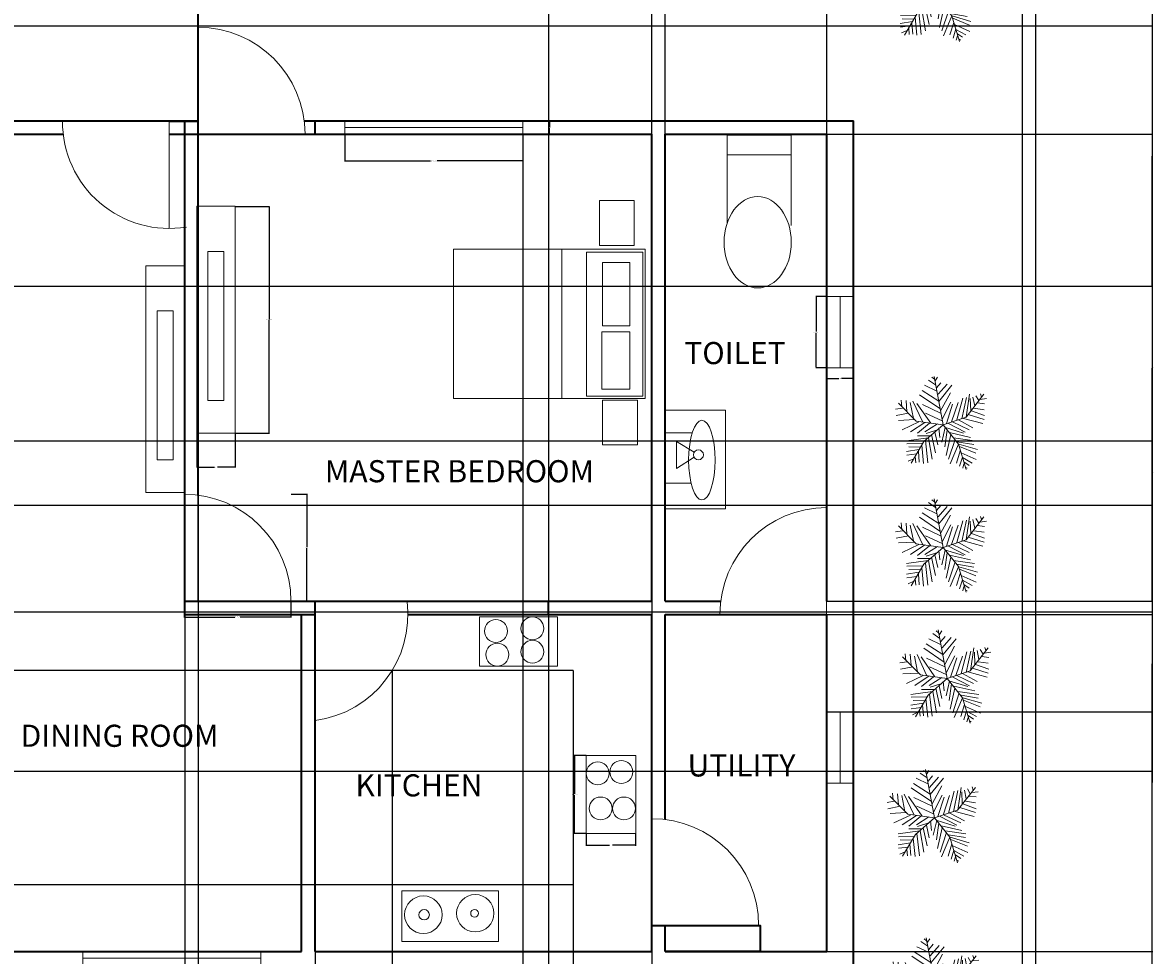
# Model space of a CAD drawing. Units: inches. Extents: x -86 to 773, y -188 to 560.
# Tile 5 of 6: x 392 to 773, y 85 to 400. Entities that reach past the tile are written whole.
import ezdxf

# ---------------------------------------------------------------- set-up
doc = ezdxf.new("R2010")
doc.units = ezdxf.units.IN
doc.header["$MEASUREMENT"] = 0
for name, color, linetype, lineweight in [('A-ANNO-DIMS', 2, 'Continuous', 18), ('A-AREA-IDEN', 7, 'Continuous', 25), ('A-DOOR', 7, 'Continuous', 18), ('A-EQPM', 8, 'Continuous', 18), ('A-FLOR-CASE', 8, 'Continuous', 18), ('A-FLOR-FIXT', 8, 'Continuous', 18), ('A-FURN', 8, 'Continuous', 18), ('A-GLAZ', 7, 'Continuous', 18), ('A-WALL', 7, 'Continuous', 35), ('C-PROP', 7, 'Continuous', 25), ('L-HRDS', 7, 'Continuous', 18), ('L-PLNT-TREE', 8, 'Continuous', 9)]:
    doc.layers.add(name, color=color, linetype=linetype, lineweight=lineweight)
doc.styles.get("Standard").update_dxf_attribs({"font": 'arial.ttf'})
doc.dimstyles.get("Standard").update_dxf_attribs({"dimtxt": 0.18, "dimasz": 0.18, "dimexe": 0.18, "dimexo": 0.0625, "dimgap": 0.09, "dimtad": 0, "dimtih": 1, "dimtoh": 1, "dimdec": 4, "dimzin": 0, "dimdsep": 46, "dimtxsty": 'Standard', "dimcen": 0.09, "dimadec": 0, "dimazin": 0, "dimtfac": 1, "dimtdec": 4, "dimtofl": 0, "dimtmove": 0, "dimatfit": 3, "dimfxl": 1, "dimtolj": 1, "dimtzin": 0, "dimarcsym": 0})

# ---------------------------------------------------------------- blocks, each defined once
blk = doc.blocks.new('Trees - Metric')
for p, q in [((-258.7244, 1362.456), (-332.3336, 1421.4348)), ((0, 0), (-266.7, 1447.8)), ((-231.1146, 1315.2628), (-166.7002, 1421.4348)), ((-129.8956, 713.6638), (-626.7704, 1032.1544)), ((-185.1152, 1008.5578), (-553.1612, 1185.4942)), ((-221.9198, 1197.3052), (-433.5526, 1338.8594)), ((-194.31, 1102.9442), (-65.4812, 1256.284)), ((-148.3106, 914.1968), (118.5418, 1220.9018)), ((-129.8956, 701.8528), (265.7602, 1185.4942)), ((-1234.059, 536.7274), (-1252.4486, 737.2604)), ((-1105.2302, 725.4494), (-1077.6458, 395.1732)), ((-902.8176, 713.6638), (-617.5756, 100.2538)), ((-93.091, 489.5342), (-700.3796, 902.3858)), ((-74.7014, 418.7444), (219.7608, 961.39)), ((-28.6766, 171.0436), (228.9556, 678.2816)), ((412.9786, 147.447), (587.8068, 796.2392)), ((560.197, 182.8292), (698.2206, 819.8358)), ((685.8, 228.6), (1219.2, 914.4)), ((689.0258, 230.0224), (790.2448, 914.1968)), ((808.6344, 784.4282), (827.0494, 418.7444)), ((891.4384, 831.6214), (946.658, 572.1096)), ((983.4626, 867.0036), (1066.2666, 725.4494)), ((1112.2914, 760.8316), (1296.3144, 784.4282)), ((1121.4862, 925.9824), (1149.0706, 831.6214)), ((-1206.4492, 501.3198), (-1418.082, 465.9376)), ((-1031.621, 347.98), (-1399.667, 277.1902)), ((-800.1, 114.3), (-1333.5, 647.7)), ((-976.4268, 666.4706), (-884.4026, 194.6402)), ((-369.1382, 53.086), (-783.1836, 642.874)), ((-617.5756, 607.4918), (-74.7014, 347.98)), ((-525.5514, 347.98), (-28.6766, 123.8504)), ((100.1268, 41.275), (284.1498, 619.2774)), ((256.5654, 88.4682), (449.7832, 666.4706)), ((845.439, 418.7444), (1241.0948, 277.1902)), ((919.0482, 501.3198), (1222.6798, 454.152)), ((1029.462, 654.685), (1241.0948, 631.0884)), ((-847.598, 159.2326), (-1326.0578, 135.636)), ((-718.7946, 88.4682), (-1215.644, -147.447)), ((-543.9664, 76.6572), (-967.2066, -206.4512)), ((0, 0), (-800.1, 114.3)), ((-405.9428, 53.086), (-764.794, -241.8334)), ((0, 0), (-571.5, -495.3)), ((-166.7002, 29.4894), (-543.9664, -206.4512)), ((0, 0), (685.8, 228.6)), ((0, 0), (457.2, -571.5)), ((164.5412, 41.275), (661.416, -218.2368)), ((284.1498, 88.4682), (781.0246, -147.447)), ((458.978, 147.447), (891.4384, -88.4682)), ((615.4166, 194.6402), (1185.8752, 41.275)), ((753.4148, 312.5978), (1222.6798, 159.2326)), ((-387.5278, -324.4088), (-764.794, -324.4088)), ((-166.7002, -147.447), (-507.1618, -253.619)), ((-341.5284, -289.0012), (-221.9198, -831.6214)), ((-240.3094, -218.2368), (-157.5054, -595.7062)), ((-120.7008, -88.4682), (-93.091, -371.5766)), ((63.3222, -76.6826), (-37.8714, -513.1308)), ((44.9326, -64.897), (615.4166, -241.8334)), ((127.7366, -159.258), (54.1274, -654.685)), ((228.9556, -289.0012), (90.932, -914.1968)), ((192.151, -230.0224), (817.8292, -371.5766)), ((-442.7474, -383.3876), (-1086.8406, -477.7486)), ((-617.5756, -548.5384), (-1077.6458, -560.324)), ((-681.9646, -666.496), (-1022.4262, -654.685)), ((-571.5, -495.3), (-952.5, -1143)), ((-635.9652, -607.5172), (-580.771, -1150.1374)), ((-525.5514, -465.963), (-451.9422, -1126.5408)), ((-433.5526, -383.3876), (-323.1134, -1020.3688)), ((357.759, -430.5554), (164.5412, -1020.3688)), ((458.978, -572.1096), (210.5406, -1161.923)), ((311.7596, -383.3876), (937.4378, -477.7486)), ((412.9786, -501.3452), (919.0482, -583.9206)), ((457.2, -571.5), (685.8, -1333.5)), ((468.1982, -572.1096), (1029.462, -737.2604)), ((486.5878, -642.8994), (983.4626, -843.4324)), ((-718.7946, -737.2604), (-1086.8406, -796.2392)), ((-783.1836, -867.029), (-1077.6458, -902.4112)), ((-875.2078, -1008.5832), (-1040.8412, -1079.3476)), ((-829.2084, -937.7934), (-810.7934, -1126.5408)), ((-737.1842, -784.4536), (-709.5744, -1114.7298)), ((514.1976, -772.6426), (403.7838, -1138.3264)), ((578.612, -961.39), (495.7826, -1232.7128)), ((541.8074, -831.6214), (992.6574, -1032.1544)), ((578.612, -973.1756), (873.0488, -1138.3264)), ((624.6114, -1161.923), (587.8068, -1291.6916)), ((624.6114, -1102.9442), (781.0246, -1209.1162)), ((679.8056, -1268.095), (716.6102, -1291.6916))]:
    blk.add_line(p, q)
blk = doc.blocks.new('BED-DOUBLE-NIGHTSTANDS')
blk.add_line((16.69, 36.48), (66.76, 36.48))
for points in [[(16.43, 64.62), (66.76, 64.62), (66.76, 0), (16.43, 0)], [(17.47, 63.83), (65.98, 63.83), (65.98, 44.81), (17.47, 44.81)], [(82.41, 62.01), (67.29, 62.01), (67.29, 50.29), (82.41, 50.29)], [(15.13, 60.97), (0, 60.97), (0, 49.24), (15.13, 49.24)], [(20.86, 59.41), (42.25, 59.41), (42.25, 50.29), (20.86, 50.29)], [(44.34, 59.41), (63.63, 59.41), (63.63, 50.03), (44.34, 50.03)]]:
    blk.add_lwpolyline(points, close=True)
blk = doc.blocks.new('DOOR-SWING-36')
for p, q in [((0, 0), (0, 36)), ((36, 0), (0, 0))]:
    blk.add_line(p, q)
blk.add_arc((0, 0), 36, 0, 90)
blk = doc.blocks.new('DOOR-LEAF-36')
blk.add_line((0, 0), (36, 0))
blk.add_arc((36, 0), 36, 90, 180)
blk = doc.blocks.new('WIN-24-W9')
for p, q in [((0, 9), (0, 0)), ((24, 9), (24, 0)), ((24, 4.5), (0, 4.5))]:
    blk.add_line(p, q)
blk = doc.blocks.new('WIN-60-W4_5')
for p, q in [((0, 4.5), (0, 0)), ((60, 4.5), (60, 0)), ((60, 2.25), (0, 2.25))]:
    blk.add_line(p, q)
blk = doc.blocks.new('COOKTOP-4-BURNER')
blk.add_lwpolyline([(0, 16.64), (26.31, 16.64), (26.31, 0), (0, 0)], close=True)
for centre in [(5.55, 11.81), (17.86, 12.69), (6.03, 3.86), (17.86, 4.82)]:
    blk.add_circle(centre, 3.86)
blk = doc.blocks.new('MEDIA-CONSOLE')
for points in [[(0, 76.46), (12.95, 76.46), (12.95, 0), (0, 0)], [(3.81, 61.24), (9.14, 61.24), (9.14, 11.03), (3.81, 11.03)]]:
    blk.add_lwpolyline(points, close=True)
blk = doc.blocks.new('BASIN-TAP')
blk.add_lwpolyline([(3.11, 5.27), (9.09, 9.11), (9.09, 0), (3.06, 3.55)])
blk.add_circle((1.66, 4.45), 1.66)
blk = doc.blocks.new('*D25')
at = {"layer": 'A-ANNO-DIMS', "color": 0, "lineweight": -2, "transparency": 16777216}
for p, q in [((446.27, 204.59), (446.27, 199.07)), ((482.27, 204.59), (482.27, 199.07)), ((446.45, 199.25), (463.34, 199.25)), ((482.09, 199.25), (465.21, 199.25))]:
    blk.add_line(p, q, dxfattribs=at)
at = {"layer": 'A-ANNO-DIMS', "color": 0, "transparency": 16777216}
for points in [[(446.45, 199.28), (446.45, 199.22), (446.27, 199.25)], [(482.09, 199.28), (482.09, 199.22), (482.27, 199.25)]]:
    blk.add_solid(points, dxfattribs=at)
at = {"layer": 'Defpoints', "color": 0, "transparency": 16777216}
for p in [(446.27, 204.65), (482.27, 204.65), (482.27, 199.25)]:
    blk.add_point(p, dxfattribs=at)
at = {"layer": 'A-ANNO-DIMS', "color": 0, "transparency": 16777216, "insert": (464.27, 199.25), "char_height": 0.18, "attachment_point": 5}
blk.add_mtext('\\A1;DOOR 36 TYP.', dxfattribs=at)
blk = doc.blocks.new('*D26')
at = {"layer": 'A-ANNO-DIMS', "color": 0, "lineweight": -2, "transparency": 16777216}
for p, q in [((482.34, 240.65), (487.85, 240.65)), ((487.67, 240.47), (487.67, 222.83)), ((487.67, 204.83), (487.67, 222.47)), ((482.34, 204.65), (487.85, 204.65))]:
    blk.add_line(p, q, dxfattribs=at)
at = {"layer": 'A-ANNO-DIMS', "color": 0, "transparency": 16777216}
for points in [[(487.64, 240.47), (487.7, 240.47), (487.67, 240.65)], [(487.64, 204.83), (487.7, 204.83), (487.67, 204.65)]]:
    blk.add_solid(points, dxfattribs=at)
at = {"layer": 'Defpoints', "color": 0, "transparency": 16777216}
for p in [(482.27, 240.65), (487.67, 240.65), (482.27, 204.65)]:
    blk.add_point(p, dxfattribs=at)
at = {"layer": 'A-ANNO-DIMS', "color": 0, "transparency": 16777216, "insert": (487.67, 222.65), "char_height": 0.18, "attachment_point": 5}
blk.add_mtext('\\A1;36 TYP.', dxfattribs=at)
blk = doc.blocks.new('*D27')
at = {"layer": 'A-ANNO-DIMS', "color": 0, "lineweight": -2, "transparency": 16777216}
for p, q in [((662.95, 307.3), (659.23, 307.3)), ((659.41, 307.12), (659.41, 295.48)), ((659.41, 283.48), (659.41, 295.11)), ((662.95, 283.3), (659.23, 283.3))]:
    blk.add_line(p, q, dxfattribs=at)
at = {"layer": 'A-ANNO-DIMS', "color": 0, "transparency": 16777216}
for points in [[(659.38, 307.12), (659.44, 307.12), (659.41, 307.3)], [(659.38, 283.48), (659.44, 283.48), (659.41, 283.3)]]:
    blk.add_solid(points, dxfattribs=at)
at = {"layer": 'Defpoints', "color": 0, "transparency": 16777216}
for p in [(659.41, 307.3), (663.01, 307.3), (663.01, 283.3)]:
    blk.add_point(p, dxfattribs=at)
at = {"layer": 'A-ANNO-DIMS', "color": 0, "transparency": 16777216, "insert": (659.41, 295.3), "char_height": 0.18, "attachment_point": 5}
blk.add_mtext('\\A1;WINDOW 24 TYP.', dxfattribs=at)
blk = doc.blocks.new('*D28')
at = {"layer": 'A-ANNO-DIMS', "color": 0, "lineweight": -2, "transparency": 16777216}
for p, q in [((663.01, 283.23), (663.01, 279.52)), ((672.01, 283.23), (672.01, 279.52)), ((663.19, 279.7), (667.05, 279.7)), ((671.83, 279.7), (667.97, 279.7))]:
    blk.add_line(p, q, dxfattribs=at)
at = {"layer": 'A-ANNO-DIMS', "color": 0, "transparency": 16777216}
for points in [[(663.19, 279.73), (663.19, 279.67), (663.01, 279.7)], [(671.83, 279.73), (671.83, 279.67), (672.01, 279.7)]]:
    blk.add_solid(points, dxfattribs=at)
at = {"layer": 'Defpoints', "color": 0, "transparency": 16777216}
for p in [(663.01, 283.3), (672.01, 283.3), (663.01, 279.7)]:
    blk.add_point(p, dxfattribs=at)
at = {"layer": 'A-ANNO-DIMS', "color": 0, "transparency": 16777216, "insert": (667.51, 279.7), "char_height": 0.18, "attachment_point": 5}
blk.add_mtext('\\A1;9 TYP.', dxfattribs=at)
blk = doc.blocks.new('*D29')
at = {"layer": 'A-ANNO-DIMS', "color": 0, "lineweight": -2, "transparency": 16777216}
for p, q in [((500.48, 361.95), (500.48, 352.83)), ((560.48, 361.95), (560.48, 352.83)), ((500.66, 353.01), (529.36, 353.01)), ((560.3, 353.01), (531.59, 353.01))]:
    blk.add_line(p, q, dxfattribs=at)
at = {"layer": 'A-ANNO-DIMS', "color": 0, "transparency": 16777216}
for points in [[(500.66, 353.04), (500.66, 352.98), (500.48, 353.01)], [(560.3, 353.04), (560.3, 352.98), (560.48, 353.01)]]:
    blk.add_solid(points, dxfattribs=at)
at = {"layer": 'Defpoints', "color": 0, "transparency": 16777216}
for p in [(500.48, 362.01), (560.48, 362.01), (560.48, 353.01)]:
    blk.add_point(p, dxfattribs=at)
at = {"layer": 'A-ANNO-DIMS', "color": 0, "transparency": 16777216, "insert": (530.48, 353.01), "char_height": 0.18, "attachment_point": 5}
blk.add_mtext('\\A1;WINDOW 60 TYP.', dxfattribs=at)
blk = doc.blocks.new('*D30')
at = {"layer": 'A-ANNO-DIMS', "color": 0, "lineweight": -2, "transparency": 16777216}
for p, q in [((560.54, 366.51), (569.66, 366.51)), ((569.48, 366.33), (569.48, 364.44)), ((569.48, 362.19), (569.48, 364.08)), ((560.54, 362.01), (569.66, 362.01))]:
    blk.add_line(p, q, dxfattribs=at)
at = {"layer": 'A-ANNO-DIMS', "color": 0, "transparency": 16777216}
for points in [[(569.45, 366.33), (569.51, 366.33), (569.48, 366.51)], [(569.45, 362.19), (569.51, 362.19), (569.48, 362.01)]]:
    blk.add_solid(points, dxfattribs=at)
at = {"layer": 'Defpoints', "color": 0, "transparency": 16777216}
for p in [(560.48, 366.51), (569.48, 366.51), (560.48, 362.01)]:
    blk.add_point(p, dxfattribs=at)
at = {"layer": 'A-ANNO-DIMS', "color": 0, "transparency": 16777216, "insert": (569.48, 364.26), "char_height": 0.18, "attachment_point": 5}
blk.add_mtext('\\A1;5 TYP.', dxfattribs=at)
blk = doc.blocks.new('*D39')
at = {"layer": 'A-ANNO-DIMS', "color": 0, "lineweight": -2, "transparency": 16777216}
for p, q in [((581.81, 152.57), (577.75, 152.57)), ((577.93, 152.39), (577.93, 139.6)), ((577.93, 126.45), (577.93, 139.24)), ((581.81, 126.27), (577.75, 126.27))]:
    blk.add_line(p, q, dxfattribs=at)
at = {"layer": 'A-ANNO-DIMS', "color": 0, "transparency": 16777216}
for points in [[(577.9, 152.39), (577.96, 152.39), (577.93, 152.57)], [(577.9, 126.45), (577.96, 126.45), (577.93, 126.27)]]:
    blk.add_solid(points, dxfattribs=at)
at = {"layer": 'Defpoints', "color": 0, "transparency": 16777216}
for p in [(581.87, 152.57), (577.93, 126.27), (581.87, 126.27)]:
    blk.add_point(p, dxfattribs=at)
at = {"layer": 'A-ANNO-DIMS', "color": 0, "transparency": 16777216, "insert": (577.93, 139.42), "char_height": 0.18, "attachment_point": 5}
blk.add_mtext('\\A1;COOKTOP 26 TYP.', dxfattribs=at)
blk = doc.blocks.new('*D40')
at = {"layer": 'A-ANNO-DIMS', "color": 0, "lineweight": -2, "transparency": 16777216}
for p, q in [((581.87, 126.21), (581.87, 122.14)), ((598.51, 126.21), (598.51, 122.14)), ((582.05, 122.32), (589.67, 122.32)), ((598.33, 122.32), (590.71, 122.32))]:
    blk.add_line(p, q, dxfattribs=at)
at = {"layer": 'A-ANNO-DIMS', "color": 0, "transparency": 16777216}
for points in [[(582.05, 122.35), (582.05, 122.29), (581.87, 122.32)], [(598.33, 122.35), (598.33, 122.29), (598.51, 122.32)]]:
    blk.add_solid(points, dxfattribs=at)
at = {"layer": 'Defpoints', "color": 0, "transparency": 16777216}
for p in [(581.87, 126.27), (598.51, 126.27), (598.51, 122.32)]:
    blk.add_point(p, dxfattribs=at)
at = {"layer": 'A-ANNO-DIMS', "color": 0, "transparency": 16777216, "insert": (590.19, 122.32), "char_height": 0.18, "attachment_point": 5}
blk.add_mtext('\\A1;17 TYP.', dxfattribs=at)
blk = doc.blocks.new('*D41')
at = {"layer": 'A-ANNO-DIMS', "color": 0, "lineweight": -2, "transparency": 16777216}
for p, q in [((463.51, 337.71), (475.09, 337.71)), ((474.91, 337.53), (474.91, 299.67)), ((474.91, 261.44), (474.91, 299.3)), ((463.51, 261.26), (475.09, 261.26))]:
    blk.add_line(p, q, dxfattribs=at)
at = {"layer": 'A-ANNO-DIMS', "color": 0, "transparency": 16777216}
for points in [[(474.88, 337.53), (474.94, 337.53), (474.91, 337.71)], [(474.88, 261.44), (474.94, 261.44), (474.91, 261.26)]]:
    blk.add_solid(points, dxfattribs=at)
at = {"layer": 'Defpoints', "color": 0, "transparency": 16777216}
for p in [(463.44, 337.71), (474.91, 337.71), (463.44, 261.26)]:
    blk.add_point(p, dxfattribs=at)
at = {"layer": 'A-ANNO-DIMS', "color": 0, "transparency": 16777216, "insert": (474.91, 299.48), "char_height": 0.18, "attachment_point": 5}
blk.add_mtext('\\A1;CONSOLE 76 TYP.', dxfattribs=at)
blk = doc.blocks.new('*D42')
at = {"layer": 'A-ANNO-DIMS', "color": 0, "lineweight": -2, "transparency": 16777216}
for p, q in [((450.5, 261.19), (450.5, 249.61)), ((463.44, 261.19), (463.44, 249.61)), ((450.68, 249.79), (456.45, 249.79)), ((463.26, 249.79), (457.49, 249.79))]:
    blk.add_line(p, q, dxfattribs=at)
at = {"layer": 'A-ANNO-DIMS', "color": 0, "transparency": 16777216}
for points in [[(450.68, 249.82), (450.68, 249.76), (450.5, 249.79)], [(463.26, 249.82), (463.26, 249.76), (463.44, 249.79)]]:
    blk.add_solid(points, dxfattribs=at)
at = {"layer": 'Defpoints', "color": 0, "transparency": 16777216}
for p in [(450.5, 261.26), (463.44, 261.26), (463.44, 249.79)]:
    blk.add_point(p, dxfattribs=at)
at = {"layer": 'A-ANNO-DIMS', "color": 0, "transparency": 16777216, "insert": (456.97, 249.79), "char_height": 0.18, "attachment_point": 5}
blk.add_mtext('\\A1;13 TYP.', dxfattribs=at)
blk = doc.blocks.new('*D46')
at = {"layer": 'A-ANNO-DIMS', "color": 0, "lineweight": -2, "transparency": 16777216}
for p, q in [((733.51, 486.66), (772.88, 486.66)), ((772.7, 486.48), (772.7, 169.55)), ((772.7, -147.74), (772.7, 169.19)), ((733.51, -147.92), (772.88, -147.92))]:
    blk.add_line(p, q, dxfattribs=at)
at = {"layer": 'A-ANNO-DIMS', "color": 0, "transparency": 16777216}
for points in [[(772.67, 486.48), (772.73, 486.48), (772.7, 486.66)], [(772.67, -147.74), (772.73, -147.74), (772.7, -147.92)]]:
    blk.add_solid(points, dxfattribs=at)
at = {"layer": 'Defpoints', "color": 0, "transparency": 16777216}
for p in [(733.45, 486.66), (772.7, 486.66), (733.45, -147.92)]:
    blk.add_point(p, dxfattribs=at)
at = {"layer": 'A-ANNO-DIMS', "color": 0, "transparency": 16777216, "insert": (772.7, 169.37), "char_height": 0.18, "attachment_point": 5}
blk.add_mtext('\\A1;634.6', dxfattribs=at)
blk = doc.blocks.new('*D54')
at = {"layer": 'A-ANNO-DIMS', "color": 0, "lineweight": -2, "transparency": 16777216}
for p, q in [((451.03, 440.67), (451.03, -187.76)), ((569.11, 440.67), (569.11, -187.76)), ((451.21, -187.58), (509.62, -187.58)), ((568.93, -187.58), (510.53, -187.58))]:
    blk.add_line(p, q, dxfattribs=at)
at = {"layer": 'A-ANNO-DIMS', "color": 0, "transparency": 16777216}
for points in [[(451.21, -187.55), (451.21, -187.61), (451.03, -187.58)], [(568.93, -187.55), (568.93, -187.61), (569.11, -187.58)]]:
    blk.add_solid(points, dxfattribs=at)
at = {"layer": 'Defpoints', "color": 0, "transparency": 16777216}
for p in [(451.03, 440.74), (569.11, 440.74), (569.11, -187.58)]:
    blk.add_point(p, dxfattribs=at)
at = {"layer": 'A-ANNO-DIMS', "color": 0, "transparency": 16777216, "insert": (510.07, -187.58), "char_height": 0.18, "attachment_point": 5}
blk.add_mtext('\\A1;118.08', dxfattribs=at)
blk = doc.blocks.new('*D55')
at = {"layer": 'A-ANNO-DIMS', "color": 0, "lineweight": -2, "transparency": 16777216}
for p, q in [((450.97, 440.74), (-85.98, 440.74)), ((-85.8, 440.56), (-85.8, 403.81)), ((-85.8, 366.7), (-85.8, 403.45)), ((450.97, 366.52), (-85.98, 366.52))]:
    blk.add_line(p, q, dxfattribs=at)
at = {"layer": 'A-ANNO-DIMS', "color": 0, "transparency": 16777216}
for points in [[(-85.83, 440.56), (-85.77, 440.56), (-85.8, 440.74)], [(-85.83, 366.7), (-85.77, 366.7), (-85.8, 366.52)]]:
    blk.add_solid(points, dxfattribs=at)
at = {"layer": 'Defpoints', "color": 0, "transparency": 16777216}
for p in [(451.03, 440.74), (-85.8, 366.52), (451.03, 366.52)]:
    blk.add_point(p, dxfattribs=at)
at = {"layer": 'A-ANNO-DIMS', "color": 0, "transparency": 16777216, "insert": (-85.8, 403.63), "char_height": 0.18, "attachment_point": 5}
blk.add_mtext('\\A1;74.22', dxfattribs=at)
blk = doc.blocks.new('*D61')
at = {"layer": 'A-ANNO-DIMS', "color": 0, "lineweight": -2, "transparency": 16777216}
for p, q in [((210.31, 398.62), (772.88, 398.62)), ((772.7, 398.44), (772.7, 354.88)), ((772.7, 310.95), (772.7, 354.52)), ((210.31, 310.77), (772.88, 310.77))]:
    blk.add_line(p, q, dxfattribs=at)
at = {"layer": 'A-ANNO-DIMS', "color": 0, "transparency": 16777216}
for points in [[(772.67, 398.44), (772.73, 398.44), (772.7, 398.62)], [(772.67, 310.95), (772.73, 310.95), (772.7, 310.77)]]:
    blk.add_solid(points, dxfattribs=at)
at = {"layer": 'Defpoints', "color": 0, "transparency": 16777216}
for p in [(210.25, 398.62), (210.25, 310.77), (772.7, 310.77)]:
    blk.add_point(p, dxfattribs=at)
at = {"layer": 'A-ANNO-DIMS', "color": 0, "transparency": 16777216, "insert": (772.7, 354.7), "char_height": 0.18, "attachment_point": 5}
blk.add_mtext('\\A1;87.85', dxfattribs=at)
blk = doc.blocks.new('*D62')
at = {"layer": 'A-ANNO-DIMS', "color": 0, "lineweight": -2, "transparency": 16777216}
for p, q in [((210.33, 201.01), (772.88, 201.01)), ((772.7, 200.83), (772.7, 174.33)), ((772.7, 147.46), (772.7, 173.96)), ((210.31, 147.28), (772.88, 147.28))]:
    blk.add_line(p, q, dxfattribs=at)
at = {"layer": 'A-ANNO-DIMS', "color": 0, "transparency": 16777216}
for points in [[(772.67, 200.83), (772.73, 200.83), (772.7, 201.01)], [(772.67, 147.46), (772.73, 147.46), (772.7, 147.28)]]:
    blk.add_solid(points, dxfattribs=at)
at = {"layer": 'Defpoints', "color": 0, "transparency": 16777216}
for p in [(210.26, 201.01), (210.25, 147.28), (772.7, 147.28)]:
    blk.add_point(p, dxfattribs=at)
at = {"layer": 'A-ANNO-DIMS', "color": 0, "transparency": 16777216, "insert": (772.7, 174.14), "char_height": 0.18, "attachment_point": 5}
blk.add_mtext('\\A1;53.72', dxfattribs=at)
blk = doc.blocks.new('*D65')
at = {"layer": 'A-ANNO-DIMS', "color": 0, "lineweight": -2, "transparency": 16777216}
for p, q in [((446.53, 366.45), (446.53, -187.76)), ((215.06, 361.95), (215.06, -187.76)), ((215.24, -187.58), (330.33, -187.58)), ((446.35, -187.58), (331.26, -187.58))]:
    blk.add_line(p, q, dxfattribs=at)
at = {"layer": 'A-ANNO-DIMS', "color": 0, "transparency": 16777216}
for points in [[(215.24, -187.55), (215.24, -187.61), (215.06, -187.58)], [(446.35, -187.55), (446.35, -187.61), (446.53, -187.58)]]:
    blk.add_solid(points, dxfattribs=at)
at = {"layer": 'Defpoints', "color": 0, "transparency": 16777216}
for p in [(446.53, 366.52), (215.06, 362.02), (446.53, -187.58)]:
    blk.add_point(p, dxfattribs=at)
at = {"layer": 'A-ANNO-DIMS', "color": 0, "transparency": 16777216, "insert": (330.8, -187.58), "char_height": 0.18, "attachment_point": 5}
blk.add_mtext('\\A1;231.47', dxfattribs=at)
blk = doc.blocks.new('*D67')
at = {"layer": 'A-ANNO-DIMS', "color": 0, "lineweight": -2, "transparency": 16777216}
for p, q in [((451.03, 204.72), (451.03, 560.19)), ((451.21, 560.01), (527.05, 560.01)), ((603.79, 560.01), (527.96, 560.01)), ((603.97, 204.64), (603.97, 560.19))]:
    blk.add_line(p, q, dxfattribs=at)
at = {"layer": 'A-ANNO-DIMS', "color": 0, "transparency": 16777216}
for points in [[(451.21, 560.04), (451.21, 559.98), (451.03, 560.01)], [(603.79, 560.04), (603.79, 559.98), (603.97, 560.01)]]:
    blk.add_solid(points, dxfattribs=at)
at = {"layer": 'Defpoints', "color": 0, "transparency": 16777216}
for p in [(603.97, 560.01), (451.03, 204.65), (603.97, 204.58)]:
    blk.add_point(p, dxfattribs=at)
at = {"layer": 'A-ANNO-DIMS', "color": 0, "transparency": 16777216, "insert": (527.5, 560.01), "char_height": 0.18, "attachment_point": 5}
blk.add_mtext('\\A1;152.94', dxfattribs=at)
blk = doc.blocks.new('*D68')
at = {"layer": 'A-ANNO-DIMS', "color": 0, "lineweight": -2, "transparency": 16777216}
for p, q in [((608.47, 362.08), (608.47, 560.19)), ((608.65, 560.01), (635.35, 560.01)), ((662.83, 560.01), (636.13, 560.01)), ((663.01, 362.08), (663.01, 560.19))]:
    blk.add_line(p, q, dxfattribs=at)
at = {"layer": 'A-ANNO-DIMS', "color": 0, "transparency": 16777216}
for points in [[(608.65, 560.04), (608.65, 559.98), (608.47, 560.01)], [(662.83, 560.04), (662.83, 559.98), (663.01, 560.01)]]:
    blk.add_solid(points, dxfattribs=at)
at = {"layer": 'Defpoints', "color": 0, "transparency": 16777216}
for p in [(663.01, 560.01), (608.47, 362.02), (663.01, 362.02)]:
    blk.add_point(p, dxfattribs=at)
at = {"layer": 'A-ANNO-DIMS', "color": 0, "transparency": 16777216, "insert": (635.74, 560.01), "char_height": 0.18, "attachment_point": 5}
blk.add_mtext('\\A1;54.54', dxfattribs=at)
blk = doc.blocks.new('*D69')
at = {"layer": 'A-ANNO-DIMS', "color": 0, "lineweight": -2, "transparency": 16777216}
for p, q in [((663.07, 362.02), (772.88, 362.02)), ((772.7, 361.84), (772.7, 283.48)), ((772.7, 204.76), (772.7, 283.11)), ((663.07, 204.58), (772.88, 204.58))]:
    blk.add_line(p, q, dxfattribs=at)
at = {"layer": 'A-ANNO-DIMS', "color": 0, "transparency": 16777216}
for points in [[(772.67, 361.84), (772.73, 361.84), (772.7, 362.02)], [(772.67, 204.76), (772.73, 204.76), (772.7, 204.58)]]:
    blk.add_solid(points, dxfattribs=at)
at = {"layer": 'Defpoints', "color": 0, "transparency": 16777216}
for p in [(663.01, 362.02), (663.01, 204.58), (772.7, 204.58)]:
    blk.add_point(p, dxfattribs=at)
at = {"layer": 'A-ANNO-DIMS', "color": 0, "transparency": 16777216, "insert": (772.7, 283.3), "char_height": 0.18, "attachment_point": 5}
blk.add_mtext('\\A1;157.44', dxfattribs=at)
blk = doc.blocks.new('*D70')
at = {"layer": 'A-ANNO-DIMS', "color": 0, "lineweight": -2, "transparency": 16777216}
for p, q in [((663.07, 200.08), (772.88, 200.08)), ((772.7, 199.9), (772.7, 143.47)), ((772.7, 86.68), (772.7, 143.1)), ((663.07, 86.5), (772.88, 86.5))]:
    blk.add_line(p, q, dxfattribs=at)
at = {"layer": 'A-ANNO-DIMS', "color": 0, "transparency": 16777216}
for points in [[(772.67, 199.9), (772.73, 199.9), (772.7, 200.08)], [(772.67, 86.68), (772.73, 86.68), (772.7, 86.5)]]:
    blk.add_solid(points, dxfattribs=at)
at = {"layer": 'Defpoints', "color": 0, "transparency": 16777216}
for p in [(663.01, 200.08), (663.01, 86.5), (772.7, 86.5)]:
    blk.add_point(p, dxfattribs=at)
at = {"layer": 'A-ANNO-DIMS', "color": 0, "transparency": 16777216, "insert": (772.7, 143.29), "char_height": 0.18, "attachment_point": 5}
blk.add_mtext('\\A1;113.58', dxfattribs=at)
blk = doc.blocks.new('*D71')
at = {"layer": 'A-ANNO-DIMS', "color": 0, "lineweight": -2, "transparency": 16777216}
for p, q in [((490.39, 86.43), (490.39, 47.07)), ((603.97, 86.43), (603.97, 47.07)), ((490.57, 47.25), (546.73, 47.25)), ((603.79, 47.25), (547.64, 47.25))]:
    blk.add_line(p, q, dxfattribs=at)
at = {"layer": 'A-ANNO-DIMS', "color": 0, "transparency": 16777216}
for points in [[(490.57, 47.28), (490.57, 47.22), (490.39, 47.25)], [(603.79, 47.28), (603.79, 47.22), (603.97, 47.25)]]:
    blk.add_solid(points, dxfattribs=at)
at = {"layer": 'Defpoints', "color": 0, "transparency": 16777216}
for p in [(490.39, 86.5), (603.97, 86.5), (490.39, 47.25)]:
    blk.add_point(p, dxfattribs=at)
at = {"layer": 'A-ANNO-DIMS', "color": 0, "transparency": 16777216, "insert": (547.18, 47.25), "char_height": 0.18, "attachment_point": 5}
blk.add_mtext('\\A1;113.58', dxfattribs=at)
blk = doc.blocks.new('*D72')
at = {"layer": 'A-ANNO-DIMS', "color": 0, "lineweight": -2, "transparency": 16777216}
for p, q in [((560.48, 361.95), (560.48, -187.76)), ((603.97, 361.95), (603.97, -187.76)), ((560.66, -187.58), (581.76, -187.58)), ((603.79, -187.58), (582.69, -187.58))]:
    blk.add_line(p, q, dxfattribs=at)
at = {"layer": 'A-ANNO-DIMS', "color": 0, "transparency": 16777216}
for points in [[(560.66, -187.55), (560.66, -187.61), (560.48, -187.58)], [(603.79, -187.55), (603.79, -187.61), (603.97, -187.58)]]:
    blk.add_solid(points, dxfattribs=at)
at = {"layer": 'Defpoints', "color": 0, "transparency": 16777216}
for p in [(560.48, 362.01), (603.97, 362.02), (603.97, -187.58)]:
    blk.add_point(p, dxfattribs=at)
at = {"layer": 'A-ANNO-DIMS', "color": 0, "transparency": 16777216, "insert": (582.22, -187.58), "char_height": 0.18, "attachment_point": 5}
blk.add_mtext('\\A1;43.496', dxfattribs=at)
blk = doc.blocks.new('*D73')
at = {"layer": 'A-ANNO-DIMS', "color": 0, "lineweight": -2, "transparency": 16777216}
for p, q in [((577.4, 181.27), (-85.98, 181.27)), ((-85.8, 181.09), (-85.8, 145.29)), ((-85.8, 109.12), (-85.8, 144.92)), ((577.4, 108.94), (-85.98, 108.94))]:
    blk.add_line(p, q, dxfattribs=at)
at = {"layer": 'A-ANNO-DIMS', "color": 0, "transparency": 16777216}
for points in [[(-85.83, 181.09), (-85.77, 181.09), (-85.8, 181.27)], [(-85.83, 109.12), (-85.77, 109.12), (-85.8, 108.94)]]:
    blk.add_solid(points, dxfattribs=at)
at = {"layer": 'Defpoints', "color": 0, "transparency": 16777216}
for p in [(-85.8, 181.27), (577.46, 181.27), (577.46, 108.94)]:
    blk.add_point(p, dxfattribs=at)
at = {"layer": 'A-ANNO-DIMS', "color": 0, "transparency": 16777216, "insert": (-85.8, 145.11), "char_height": 0.18, "attachment_point": 5}
blk.add_mtext('\\A1;72.33', dxfattribs=at)
blk = doc.blocks.new('*D74')
at = {"layer": 'A-ANNO-DIMS', "color": 0, "lineweight": -2, "transparency": 16777216}
for p, q in [((516.4, 181.21), (516.4, -187.76)), ((577.46, 181.21), (577.46, -187.76)), ((516.58, -187.58), (546.54, -187.58)), ((577.28, -187.58), (547.32, -187.58))]:
    blk.add_line(p, q, dxfattribs=at)
at = {"layer": 'A-ANNO-DIMS', "color": 0, "transparency": 16777216}
for points in [[(516.58, -187.55), (516.58, -187.61), (516.4, -187.58)], [(577.28, -187.55), (577.28, -187.61), (577.46, -187.58)]]:
    blk.add_solid(points, dxfattribs=at)
at = {"layer": 'Defpoints', "color": 0, "transparency": 16777216}
for p in [(516.4, 181.27), (577.46, 181.27), (577.46, -187.58)]:
    blk.add_point(p, dxfattribs=at)
at = {"layer": 'A-ANNO-DIMS', "color": 0, "transparency": 16777216, "insert": (546.93, -187.58), "char_height": 0.18, "attachment_point": 5}
blk.add_mtext('\\A1;61.06', dxfattribs=at)
blk = doc.blocks.new('*D79')
at = {"layer": 'A-ANNO-DIMS', "color": 0, "lineweight": -2, "transparency": 16777216}
for p, q in [((210.31, 258.61), (772.88, 258.61)), ((772.7, 258.43), (772.7, 247.99)), ((772.7, 237.19), (772.7, 247.63)), ((210.33, 237.01), (772.88, 237.01))]:
    blk.add_line(p, q, dxfattribs=at)
at = {"layer": 'A-ANNO-DIMS', "color": 0, "transparency": 16777216}
for points in [[(772.67, 258.43), (772.73, 258.43), (772.7, 258.61)], [(772.67, 237.19), (772.73, 237.19), (772.7, 237.01)]]:
    blk.add_solid(points, dxfattribs=at)
at = {"layer": 'Defpoints', "color": 0, "transparency": 16777216}
for p in [(210.24, 258.61), (210.26, 237.01), (772.7, 237.01)]:
    blk.add_point(p, dxfattribs=at)
at = {"layer": 'A-ANNO-DIMS', "color": 0, "transparency": 16777216, "insert": (772.7, 247.81), "char_height": 0.18, "attachment_point": 5}
blk.add_mtext('\\A1;21.604', dxfattribs=at)
blk = doc.blocks.new('*D80')
at = {"layer": 'A-ANNO-DIMS', "color": 0, "lineweight": -2, "transparency": 16777216}
for p, q in [((663.07, 200.08), (772.88, 200.08)), ((772.7, 199.9), (772.7, 183.86)), ((772.7, 167.47), (772.7, 183.5)), ((663.07, 167.29), (772.88, 167.29))]:
    blk.add_line(p, q, dxfattribs=at)
at = {"layer": 'A-ANNO-DIMS', "color": 0, "transparency": 16777216}
for points in [[(772.67, 199.9), (772.73, 199.9), (772.7, 200.08)], [(772.67, 167.47), (772.73, 167.47), (772.7, 167.29)]]:
    blk.add_solid(points, dxfattribs=at)
at = {"layer": 'Defpoints', "color": 0, "transparency": 16777216}
for p in [(663.01, 200.08), (772.7, 200.08), (663.01, 167.29)]:
    blk.add_point(p, dxfattribs=at)
at = {"layer": 'A-ANNO-DIMS', "color": 0, "transparency": 16777216, "insert": (772.7, 183.68), "char_height": 0.18, "attachment_point": 5}
blk.add_mtext('\\A1;32.79', dxfattribs=at)

msp = doc.modelspace()

# ---------------------------------------------------------------- linework, layer by layer
at = {"layer": 'A-DOOR'}
for p, q in [((441.2175, 330.2481), (441.2175, 366.2481)), ((451.0315, 366.2481), (441.2175, 366.2481)), ((485.8915, 200.0476), (485.7062, 200.0476)), ((485.7062, 200.0476), (485.7062, 164.0476))]:
    msp.add_line(p, q, dxfattribs=at)
msp.add_lwpolyline([(603.9715, 95.2638), (639.9715, 95.2638), (639.9715, 95.2638), (603.9715, 95.2638)], close=True, dxfattribs=at)
for centre, start, end in [((441.2367, 366.2481), 179.572446, 279.293446), ((485.7062, 200.0476), 277.477995, 7.227475), ((485.7062, 200.0476), 270, 270.294812)]:
    msp.add_arc(centre, 36, start, end, dxfattribs=at)
at = {"layer": 'A-FLOR-CASE'}
for p, q in [((516.4009, 181.2736), (577.46, 181.2736)), ((577.46, 181.2736), (577.46, 108.94)), ((577.46, 108.94), (490.3362, 108.94))]:
    msp.add_line(p, q, dxfattribs=at)
at = {"layer": 'A-FLOR-FIXT'}
for p, q in [((629.3677, 332.1856), (629.3677, 361.7542)), ((650.9673, 361.7542), (629.3677, 361.7542)), ((650.9673, 331.2317), (650.9673, 361.7542)), ((629.3677, 355.0774), (650.9673, 355.0774))]:
    msp.add_line(p, q, dxfattribs=at)
for points in [[(608.6206, 269.023), (628.7694, 269.023), (628.7694, 235.7121), (608.6206, 235.7121)], [(519.6388, 106.9), (552.2072, 106.9), (552.2072, 89.9028), (519.6388, 89.9028)]]:
    msp.add_lwpolyline(points, close=True, dxfattribs=at)
msp.add_lwpolyline([(617.1997, 244.3972), (608.5983, 244.3972), (608.5983, 261.3447), (617.5851, 261.3447)], dxfattribs=at)
for centre, radius in [((526.9302, 98.887), 6.3337), ((544.4297, 99.3727), 6.3043), ((527.1732, 98.887), 1.7679), ((544.1866, 99.3727), 1.3078)]:
    msp.add_circle(centre, radius, dxfattribs=at)
for centre, major_axis, ratio in [((639.6614, 325.6016), (0, 15.3922), 0.73614587), ((620.8497, 252.1648), (0, -13.4168), 0.33364881)]:
    msp.add_ellipse(centre, major_axis=major_axis, ratio=ratio, dxfattribs=at)
at = {"layer": 'A-WALL'}
for p, q in [((451.0315, 240.3369), (451.0315, 440.7367)), ((446.5315, 240.6517), (446.5315, 366.5167)), ((490.3915, 362.0167), (490.3915, 366.5167)), ((672.0115, -143.4172), (672.0115, 366.5167)), ((485.8915, 362.0167), (485.8915, 362.0673)), ((603.9715, 204.5767), (603.9715, 362.0167)), ((608.4715, 204.5767), (608.4715, 362.0167)), ((663.0115, 204.5767), (663.0115, 362.0167)), ((446.5315, 200.0767), (446.5315, 204.6526)), ((451.0315, 204.5767), (451.0315, 204.6526)), ((490.3915, 86.4967), (490.3915, 204.5767)), ((569.1115, 200.0767), (569.1115, 204.5767)), ((485.8915, 86.4967), (485.8915, 200.0767)), ((603.9715, 86.4967), (603.9715, 200.0767)), ((608.4715, 130.9814), (608.4715, 200.0767)), ((663.0115, 86.4967), (663.0115, 200.0767)), ((608.4715, 86.4967), (608.4715, 95.2638))]:
    msp.add_line(p, q, dxfattribs=at)
for points in [[(215.0615, 366.5167), (451.0315, 366.5167)], [(486.7503, 366.5167), (672.0115, 366.5167)], [(215.0615, 362.0167), (405.4862, 362.0167)], [(441.2175, 362.0167), (603.9715, 362.0167)], [(608.4715, 362.0167), (663.0115, 362.0167)], [(446.5315, 204.5767), (603.9715, 204.5767)], [(608.4715, 204.5767), (627.1862, 204.5767)], [(662.9125, 204.5767), (663.0115, 204.5767)], [(446.5315, 200.0767), (490.3915, 200.0767)], [(521.7062, 200.0767), (603.9715, 200.0767)], [(608.4715, 200.0767), (663.0115, 200.0767)], [(603.9715, 86.4967), (603.9715, 95.2638), (640.4618, 95.2638), (640.4618, 86.4967), (608.4715, 86.4967)], [(365.392, 86.4967), (485.8915, 86.4967)], [(490.3915, 86.4967), (603.9715, 86.4967)], [(608.4715, 86.4967), (663.0115, 86.4967)]]:
    msp.add_lwpolyline(points, dxfattribs=at)
at = {"layer": 'C-PROP'}
for p, q in [((733.4515, -147.9172), (733.4515, 486.6589)), ((728.9515, -143.4172), (728.9515, 482.1589))]:
    msp.add_line(p, q, dxfattribs=at)
at = {"layer": 'L-HRDS'}
msp.add_line((569.1115, 366.5167), (569.1115, 440.7367), dxfattribs=at)

# ---------------------------------------------------------------- block references
at = {"layer": 'A-DOOR'}
for p in [(451.026, 362.067), (446.2741, 204.6522), (603.9711, 95.2634)]:
    msp.add_blockref('DOOR-SWING-36', p, dxfattribs=at)
at = {"layer": 'A-DOOR', "extrusion": (0, 0, -1), "zscale": -1, "rotation": 270}
msp.add_blockref('DOOR-LEAF-36', (-662.9127, 236.1453), dxfattribs=at)
at = {"layer": 'A-EQPM'}
msp.add_blockref('COOKTOP-4-BURNER', (545.844, 182.72), dxfattribs=at)
at = {"layer": 'A-EQPM', "rotation": 269.9999999999994}
msp.add_blockref('COOKTOP-4-BURNER', (581.8732, 152.575), dxfattribs=at)
at = {"layer": 'A-FLOR-FIXT', "rotation": 180}
msp.add_blockref('BASIN-TAP', (621.35, 258.3843), dxfattribs=at)
at = {"layer": 'A-FURN', "rotation": 270.0000000000001}
msp.add_blockref('BED-DOUBLE-NIGHTSTANDS', (537.0915, 339.6882), dxfattribs=at)
at = {"layer": 'A-FURN'}
for p in [(450.499, 261.255), (433.3747, 241.1904)]:
    msp.add_blockref('MEDIA-CONSOLE', p, dxfattribs=at)
at = {"layer": 'A-GLAZ'}
for p in [(500.4755, 362.0116), (412.1017, 82.0297)]:
    msp.add_blockref('WIN-60-W4_5', p, dxfattribs=at)
for p, rotation in [((672.0112, 283.2971), 89.99999999999967), ((672.0112, 143.2871), 89.99999999999957)]:
    msp.add_blockref('WIN-24-W9', p, dxfattribs=dict(at, rotation=rotation))
at = {"layer": 'L-PLNT-TREE', "xscale": 0.0112992005060107, "yscale": 0.0112992005060107, "zscale": 0.0112992005060107}
for p in [(699.932, 408.366), (702.1521, 264.0119), (702.1521, 222.6915), (703.5783, 178.5214), (699.2997, 131.5016), (699.5311, 74.7194)]:
    msp.add_blockref('Trees - Metric', p, dxfattribs=at)

# ---------------------------------------------------------------- texts
at = {"layer": 'A-AREA-IDEN'}
for s, height, p in [('TOILET', 7.45296, (614.8918, 284.5106)), ('MASTER BEDROOM', 7.452962, (493.6948, 244.6822)), ('DINING ROOM', 7.452962, (391.1114, 155.4889)), ('UTILITY', 7.45296, (615.9953, 145.4919)), ('KITCHEN', 7.45296, (503.9961, 138.7651))]:
    msp.add_text(s, height=height, dxfattribs=at).set_placement(p)

# ---------------------------------------------------------------- dimensions: what is measured, and where the dimension line sits
at = {"layer": 'A-ANNO-DIMS'}
for base, p1, p2, override, picture, middle in [((603.9715, 560.0063), (451.0315, 204.6526), (603.9715, 204.5767), {"dimdec": 2, "dimlfac": 1, "dimrnd": 0, "dimzin": 0, "dimdsep": 46, "dimlunit": 2}, '*D67', (527.5015, 560.0063)), ((663.0115, 560.0063), (608.4715, 362.0167), (663.0115, 362.0167), {"dimdec": 2, "dimlfac": 1, "dimrnd": 0, "dimzin": 0, "dimdsep": 46, "dimlunit": 2}, '*D68', (635.7415, 560.0063)), ((569.1115, -187.578), (451.0315, 440.7367), (569.1115, 440.7367), {"dimdec": 2, "dimlfac": 1, "dimrnd": 0, "dimzin": 0, "dimdsep": 46, "dimlunit": 2}, '*D54', (510.0715, -187.578)), ((446.5315, -187.578), (215.0615, 362.0167), (446.5315, 366.5167), {"dimdec": 2, "dimlfac": 1, "dimrnd": 0, "dimzin": 0, "dimdsep": 46, "dimlunit": 2}, '*D65', (330.7965, -187.578)), ((603.9715, -187.578), (560.4759, 362.0116), (603.9715, 362.0167), {"dimdec": 3, "dimlfac": 1, "dimrnd": 0, "dimzin": 0, "dimdsep": 46, "dimlunit": 2}, '*D72', (582.2237, -187.578)), ((577.46, -187.578), (516.4009, 181.2736), (577.46, 181.2736), {"dimdec": 2, "dimlfac": 1, "dimrnd": 0, "dimzin": 0, "dimdsep": 46, "dimlunit": 2}, '*D74', (546.9304, -187.578))]:
    dim = msp.add_linear_dim(base=base, p1=p1, p2=p2, dimstyle='Standard', override=override, dxfattribs=at)
    dim.commit()
    dim.dimension.update_dxf_attribs({"geometry": picture, "text_midpoint": middle})
for base, p1, p2, angle, override, picture, middle in [((772.7015, 486.6589), (733.4515, -147.9172), (733.4515, 486.6589), 90, {"dimdec": 1, "dimlfac": 1, "dimrnd": 0, "dimzin": 0, "dimdsep": 46, "dimlunit": 2}, '*D46', (772.7015, 169.3709)), ((-85.7985, 366.5167), (451.0315, 440.7367), (451.0315, 366.5167), 90, {"dimdec": 2, "dimlfac": 1, "dimrnd": 0, "dimzin": 0, "dimdsep": 46, "dimlunit": 2}, '*D55', (-85.7985, 403.6267)), ((772.7015, 310.7712), (210.2515, 398.6228), (210.2515, 310.7712), 90, {"dimdec": 2, "dimlfac": 1, "dimrnd": 0, "dimzin": 0, "dimdsep": 46, "dimlunit": 2}, '*D61', (772.7015, 354.697)), ((772.7015, 204.5767), (663.0115, 362.0167), (663.0115, 204.5767), 90, {"dimdec": 2, "dimlfac": 1, "dimrnd": 0, "dimzin": 0, "dimdsep": 46, "dimlunit": 2}, '*D69', (772.7015, 283.2967)), ((772.7015, 237.0056), (210.2444, 258.61), (210.2647, 237.0056), 90, {"dimdec": 3, "dimlfac": 1, "dimrnd": 0, "dimzin": 0, "dimdsep": 46, "dimlunit": 2}, '*D79', (772.7015, 247.8078)), ((772.7015, 147.2828), (210.2647, 201.0056), (210.2515, 147.2828), 90, {"dimdec": 2, "dimlfac": 1, "dimrnd": 0, "dimzin": 0, "dimdsep": 46, "dimlunit": 2}, '*D62', (772.7015, 174.1442)), ((772.7015, 86.4967), (663.0115, 200.0767), (663.0115, 86.4967), 90, {"dimdec": 2, "dimlfac": 1, "dimrnd": 0, "dimzin": 0, "dimdsep": 46, "dimlunit": 2}, '*D70', (772.7015, 143.2867)), ((772.7015, 200.0767), (663.0115, 167.2867), (663.0115, 200.0767), 90, {"dimdec": 2, "dimlfac": 1, "dimrnd": 0, "dimzin": 0, "dimdsep": 46, "dimlunit": 2}, '*D80', (772.7015, 183.6817)), ((-85.7985, 181.2736), (577.46, 108.94), (577.46, 181.2736), 90, {"dimdec": 2, "dimlfac": 1, "dimrnd": 0, "dimzin": 0, "dimdsep": 46, "dimlunit": 2}, '*D73', (-85.7985, 145.1068)), ((490.3915, 47.2467), (603.9715, 86.4967), (490.3915, 86.4967), 180, {"dimdec": 2, "dimlfac": 1, "dimrnd": 0, "dimzin": 0, "dimdsep": 46, "dimlunit": 2}, '*D71', (547.1815, 47.2467))]:
    dim = msp.add_linear_dim(base=base, p1=p1, p2=p2, angle=angle, dimstyle='Standard', override=override, dxfattribs=at)
    dim.commit()
    dim.dimension.update_dxf_attribs({"geometry": picture, "text_midpoint": middle})
for base, p1, p2, angle, text, picture, middle in [((569.4759401237, 366.5116243829), (560.4759401237, 362.0116243829), (560.4759401237, 366.5116243829), 90, '<> TYP.', '*D30', (569.4759401237, 364.2616243829)), ((474.9127, 337.7113), (463.4443, 261.2554), (463.4443, 337.7113), 90, 'CONSOLE <> TYP.', '*D41', (474.9127, 299.4834)), ((659.4115, 307.2967), (663.0115, 283.2967), (663.0115, 307.2967), 90, 'WINDOW <> TYP.', '*D27', (659.4115, 295.2967)), ((663.0115, 279.6967), (672.0115, 283.2967), (663.0115, 283.2967), 180, '<> TYP.', '*D28', (667.5115, 279.6967)), ((487.6745, 240.6526), (482.2745, 204.6526), (482.2745, 240.6526), 90, '<> TYP.', '*D26', (487.6745, 222.6526)), ((577.9275, 126.2685), (581.8734, 152.5746), (581.8734, 126.2685), 270, 'COOKTOP <> TYP.', '*D39', (577.9275, 139.4216))]:
    dim = msp.add_linear_dim(base=base, p1=p1, p2=p2, angle=angle, text=text, dimstyle='Standard', override={"dimdec": 0, "dimlfac": 1, "dimrnd": 0, "dimzin": 0, "dimdsep": 46, "dimlunit": 2}, dxfattribs=at)
    dim.commit()
    dim.dimension.update_dxf_attribs({"geometry": picture, "text_midpoint": middle})
for base, p1, p2, text, picture, middle in [((560.4759, 353.0116), (500.4759, 362.0116), (560.4759, 362.0116), 'WINDOW <> TYP.', '*D29', (530.4759, 353.0116)), ((463.4443, 249.7871), (450.4992, 261.2554), (463.4443, 261.2554), '<> TYP.', '*D42', (456.9718, 249.7871)), ((482.2745, 199.2526), (446.2745, 204.6526), (482.2745, 204.6526), 'DOOR <> TYP.', '*D25', (464.2745, 199.2526)), ((598.5102, 122.3226), (581.8734, 126.2685), (598.5102, 126.2685), '<> TYP.', '*D40', (590.1918, 122.3226))]:
    dim = msp.add_linear_dim(base=base, p1=p1, p2=p2, text=text, dimstyle='Standard', override={"dimdec": 0, "dimlfac": 1, "dimrnd": 0, "dimzin": 0, "dimdsep": 46, "dimlunit": 2}, dxfattribs=at)
    dim.commit()
    dim.dimension.update_dxf_attribs({"geometry": picture, "text_midpoint": middle})

doc.saveas('drawing.dxf')
